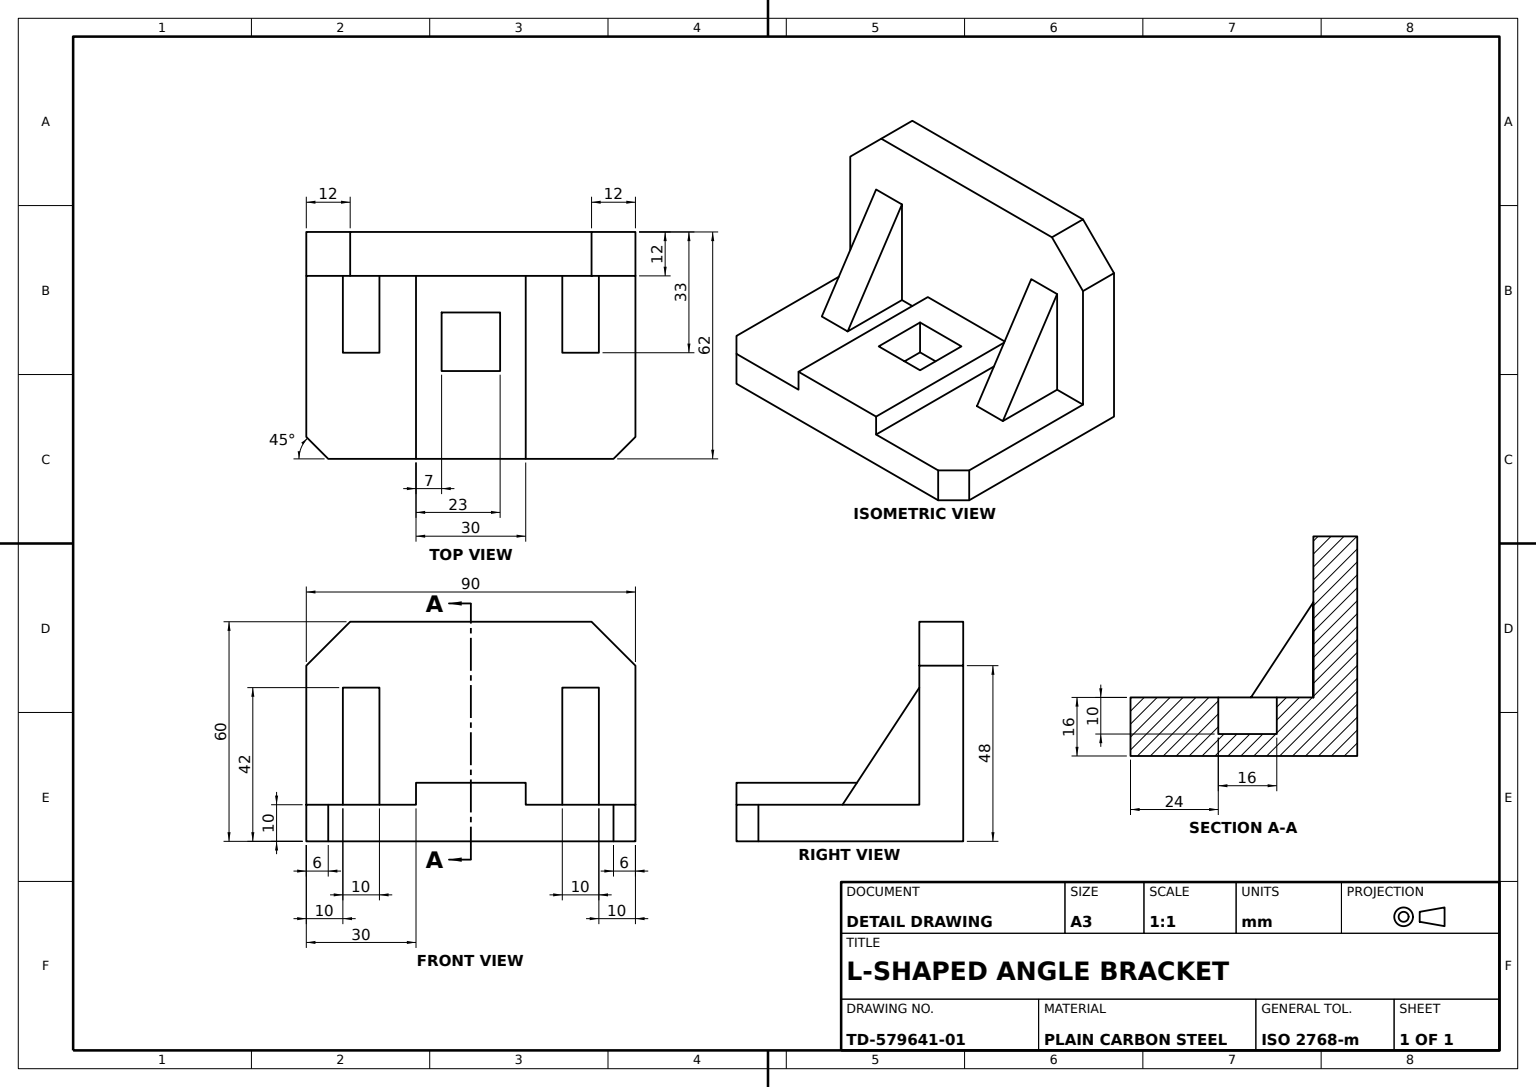
SolidWorks part; units mm, degrees
material "Plain Carbon Steel"
ref_plane "Front Plane" through (0, 0, 0) normal (0, 0, 1) x (1, 0, 0)
ref_plane "Top Plane" through (0, 0, 0) normal (0, 1, 0) x (1, 0, 0)
ref_plane "Right Plane" through (0, 0, 0) normal (1, 0, 0) x (0, 0, -1)
sketch "Bracket Profile Sketch" plane through (0, 0, 0) normal (0, 0, 1) x (1, 0, 0)
  line L0 (0, 0) -> (93.5797, 0)
  line L1 (93.5797, 0) -> (93.5797, 48)
  line L4 (81.5797, 60) -> (15.5797, 60)
  line L7 (3.5797, 48) -> (3.5797, 0)
  line L8 (3.5797, 0) -> (0, 0)
  line L9 (3.5797, 48) -> (15.5797, 60)
  line L10 (81.5797, 60) -> (93.5797, 48)
  dimension "D1" = 90
  dimension "D2" = 12
  dimension "D3" = 60
  dimension "D4" = 12
  dimension "D5" = 48
  dimension "D6" = 93.5797
extrude "Bracket Body" add sketch "Bracket Profile Sketch" along normal blind 12 contours L10 L4 L9 L7 L0 L1
sketch "Chamfered Plate Sketch" plane through (0, 0, 0) normal (0, -1, 0) x (1, 0, 0)
  line L0 (3.5797, 12) -> (3.5797, 56)
  line L1 (3.5797, 12) -> (93.5797, 12)
  line L3 (93.5797, 12) -> (93.5797, 56)
  line L6 (87.5797, 62) -> (9.5797, 62)
  line L7 (3.5797, 56) -> (9.5797, 62)
  line L8 (87.5797, 62) -> (93.5797, 56)
  dimension "D1" = 78
  dimension "D2" = 6
  dimension "D3" = 44
extrude "Chamfered Plate 78x44" add sketch "Chamfered Plate Sketch" against normal blind 10
sketch "Centre Pad Sketch" plane through (0, 10, 0) normal (0, 1, 0) x (1, 0, 0)
  line L0 (81.5797, -12) -> (15.5797, -12) construction
  line L1 (33.5797, -12) -> (63.5797, -12)
  line L2 (33.5797, -12) -> (33.5797, -62)
  line L3 (33.5797, -62) -> (63.5797, -62)
  line L4 (63.5797, -12) -> (63.5797, -62)
  line L5 (87.5797, -62) -> (9.5797, -62) construction
  line L6 (93.5797, -12) -> (93.5797, -56) construction
  dimension "D1" = 30
  dimension "D2" = 30
extrude "Centre Pad 30x30" add sketch "Centre Pad Sketch" along normal blind 6
sketch "Pad Pocket Sketch" plane through (0, 16, 0) normal (0, 1, 0) x (1, 0, 0)
  line L0 (63.5797, -12) -> (33.5797, -12) construction
  line L1 (40.5797, -22) -> (56.5797, -22)
  line L2 (40.5797, -22) -> (40.5797, -38)
  line L3 (40.5797, -38) -> (56.5797, -38)
  line L4 (56.5797, -22) -> (56.5797, -38)
  line L5 (33.5797, -12) -> (33.5797, -62) construction
  line L6 (33.5797, -12) -> (33.5797, -62) construction
  dimension "D1" = 10
  dimension "D2" = 7
  dimension "D3" = 23
extrude "Pad Pocket 10x7" cut sketch "Pad Pocket Sketch" against normal blind 10
sketch "Rib 1 Sketch" plane through (3.5797, 0, 0) normal (-1, 0, 0) x (0, 0, 1)
  line L0 (12, 10) -> (12, 42)
  line L1 (12, 48) -> (12, 10) construction
  line L2 (12, 10) -> (33, 10)
  line L3 (56, 10) -> (12, 10) construction
  line L4 (33, 10) -> (12, 42)
  line L5 (0, 48) -> (0, 0) construction
  line L6 (56, 0) -> (0, 0) construction
  dimension "D1" = 33
  dimension "D2" = 42
extrude "Gusset Rib 1" add sketch "Rib 1 Sketch" against normal blind 20
sketch "Rib 1 Trim Sketch" plane through (3.5797, 0, 0) normal (-1, 0, 0) x (0, 0, 1)
  line L0 (12, 42) -> (12, 10)
  line L1 (12, 10) -> (33, 10)
  line L2 (33, 10) -> (12, 42)
extrude "Gusset Rib 1 Trim" cut sketch "Rib 1 Trim Sketch" against normal blind 10
sketch "Rib 2 Sketch" plane through (93.5797, 0, 0) normal (1, 0, 0) x (0, 0, -1)
  line L0 (-12, 10) -> (-12, 42)
  line L1 (-12, 42) -> (-33, 10)
  line L2 (-62, 10) -> (-12, 10) construction
  line L3 (-12, 10) -> (-56, 10) construction
  line L4 (-33, 10) -> (-12, 10)
  line L5 (0, 0) -> (0, 48) construction
  dimension "D1" = 33
extrude "Gusset Rib 2" add sketch "Rib 2 Sketch" against normal blind 20
sketch "Rib 2 Trim Sketch" plane through (93.5797, 0, 0) normal (1, 0, 0) x (0, 0, -1)
  line L0 (-12, 42) -> (-12, 10)
  line L1 (-12, 10) -> (-33, 10)
  line L2 (-33, 10) -> (-12, 42)
extrude "Gusset Rib 2 Trim" cut sketch "Rib 2 Trim Sketch" against normal blind 10
